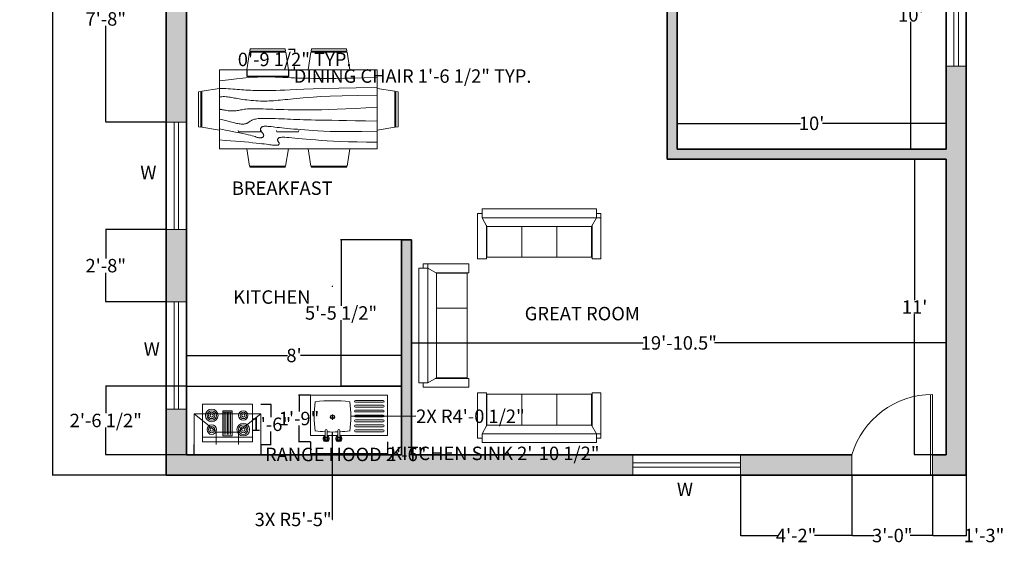
# Model space of a CAD drawing. Units: inches. Extents: x 302 to 1258, y 831 to 1373.
# Tile 1 of 13: x 302 to 742, y 836 to 1070. Entities that reach past the tile are written whole.
import ezdxf

# ---------------------------------------------------------------- set-up
doc = ezdxf.new("R2010")
doc.units = ezdxf.units.IN
doc.header["$MEASUREMENT"] = 0
for name, color, linetype, lineweight in [('A-ANNO-DIMS', 2, 'Continuous', 18), ('A-ANNO-TEXT', 7, 'Continuous', 18), ('A-AREA-IDEN', 7, 'Continuous', 18), ('A-DOOR', 3, 'Continuous', 18), ('A-EQPM', 8, 'Continuous', 18), ('A-FLOR-CASE', 8, 'Continuous', 25), ('A-FLOR-FIXT', 8, 'Continuous', 18), ('A-FURN', 8, 'Continuous', 18), ('A-GLAZ', 4, 'Continuous', 18), ('A-WALL', 7, 'Continuous', 35), ('A-WALL-PATT', 251, 'Continuous', 13)]:
    doc.layers.add(name, color=color, linetype=linetype, lineweight=lineweight)
doc.styles.get("Standard").update_dxf_attribs({"font": 'arial.ttf'})
doc.dimstyles.get("Standard").update_dxf_attribs({"dimtxt": 6, "dimasz": 0.18, "dimexe": 0.18, "dimexo": 0.0625, "dimgap": 0.09, "dimtad": 0, "dimtih": 1, "dimtoh": 1, "dimdec": 1, "dimzin": 0, "dimdsep": 46, "dimlunit": 3, "dimtxsty": 'Standard', "dimcen": 0.09, "dimadec": 0, "dimazin": 0, "dimtfac": 1, "dimtdec": 1, "dimtofl": 0, "dimtmove": 0, "dimatfit": 3, "dimfxl": 1, "dimtolj": 1, "dimtzin": 0, "dimarcsym": 0})

# ---------------------------------------------------------------- blocks, each defined once
blk = doc.blocks.new('chimmne')
for p, q in [((17.89, 6.07), (-18.11, 6.07)), ((-18.11, 6.07), (-18.11, -10.43)), ((-6.16, -3.43), (-18.11, 6.07)), ((5.94, -3.43), (17.89, 6.07)), ((17.89, 6.07), (17.89, -10.43)), ((-6.16, -3.43), (-6.16, -10.43)), ((5.94, -3.82), (-6.16, -3.82)), ((5.94, -3.43), (5.94, -10.43))]:
    blk.add_line(p, q)
for points in [[(-13.61, -9.12), (-13.61, 11.28), (13.39, 11.28), (13.39, -9.12)], [(-2.66, -5.87), (-2.66, 7.73), (2.44, 7.73), (2.44, -5.87)]]:
    blk.add_lwpolyline(points, close=True)
for points in [[(-2.66, 6.88), (2.44, 6.88)], [(-1.81, 6.88), (-1.81, -5.02)], [(-0.96, -5.02), (-0.96, 6.88)], [(-0.11, 6.88), (-0.11, -5.02)], [(0.74, -5.02), (0.74, 6.88)], [(1.59, 6.88), (1.59, -5.02)], [(13.39, -6.57), (-13.61, -6.57)]]:
    blk.add_lwpolyline(points)
for centre, radius in [((-8.55, 5.18), 3.4), ((-8.55, 5.18), 2.55), ((-8.55, 5.18), 1.7), ((-8.55, 5.18), 0.85), ((8.44, 5.18), 2.55), ((8.44, 5.18), 1.7), ((8.44, 5.18), 0.85), ((-8.55, -2.47), 2.55), ((8.44, -2.47), 3.4), ((8.44, -2.47), 2.55), ((-8.55, -2.47), 1.7), ((-8.55, -2.47), 0.85), ((8.44, -2.47), 1.7), ((8.44, -2.47), 0.85)]:
    blk.add_circle(centre, radius)
blk = doc.blocks.new('A$C799204C7')
for p, q in [((0, 34.2), (17.99, 34.2)), ((0, 0), (0, 34.2)), ((2.32, 20.01), (2.32, 32.27)), ((3.13, 20.01), (3.13, 32.27)), ((4.48, 20.01), (4.48, 32.27)), ((5.29, 20.01), (5.29, 32.27)), ((6.64, 20.01), (6.64, 32.27)), ((7.45, 20.01), (7.45, 32.27)), ((8.85, 20.01), (8.85, 32.27)), ((9.66, 20.01), (9.66, 32.27)), ((11.01, 20.01), (11.01, 32.27)), ((11.82, 20.01), (11.82, 32.27)), ((13.22, 20.01), (13.22, 32.27)), ((14.03, 20.01), (14.03, 32.27)), ((15.42, 20.01), (15.42, 32.27)), ((16.24, 20.01), (16.24, 32.27)), ((17.99, 13.08), (17.99, 34.2)), ((8.52, 9.77), (10.9, 9.77)), ((9.73, 11), (9.73, 8.54)), ((18.59, 13.08), (15.71, 13.08)), ((15.71, 12.17), (18.59, 12.17)), ((17.99, 7.36), (17.99, 12.17)), ((18.59, 7.36), (15.71, 7.36)), ((15.71, 6.45), (18.59, 6.45)), ((17.99, 0), (17.99, 6.45)), ((0, 0), (17.99, 0))]:
    blk.add_line(p, q)
for centre, radius in [((19.38, 12.62), 0.684), ((9.7, 9.77), 0.916), ((19.38, 12.62), 0.456), ((19.38, 6.91), 0.684), ((19.38, 6.91), 0.456)]:
    blk.add_circle(centre, radius)
for centre, radius, start, end in [((2.72, 32.27), 0.407, 0, 180), ((4.88, 32.27), 0.407, 0, 180), ((7.05, 32.27), 0.407, 0, 180), ((9.25, 32.27), 0.407, 0, 180), ((11.42, 32.27), 0.407, 0, 180), ((13.62, 32.27), 0.407, 0, 180), ((15.83, 32.27), 0.407, 0, 180), ((2.72, 20.01), 0.407, 180, 0), ((9.53, -30.19), 48.1, 82.3437, 97.8966), ((4.88, 20.01), 0.407, 180, 0), ((7.05, 20.01), 0.407, 180, 0), ((9.25, 20.01), 0.407, 180, 0), ((11.42, 20.01), 0.407, 180, 0), ((13.62, 20.01), 0.407, 180, 0), ((15.83, 20.01), 0.407, 180, 0), ((67.33, 9.77), 64.88, 173.1952, 186.8048), ((-48.51, 9.77), 64.88, 2.9208, 6.8048), ((19.38, 12.62), 1.37, 199.6514, 160.3603), ((19.38, 12.62), 0.911, 210.3431, 149.7554), ((15.71, 12.62), 0.456, 90, 270), ((-48.51, 9.77), 64.88, 357.8723, 2.115), ((15.71, 6.91), 0.456, 90, 270), ((-48.51, 9.77), 64.88, 353.1952, 357.0665), ((19.38, 6.91), 1.37, 199.6514, 160.3603), ((19.38, 6.91), 0.911, 210.3431, 149.7554), ((9.53, 49.73), 48.1, 262.1034, 277.6563)]:
    blk.add_arc(centre, radius, start, end)
blk = doc.blocks.new('*D11')
at = {"layer": 'A-ANNO-DIMS', "color": 0, "lineweight": -2, "transparency": 16777216}
for p, q in [((595.67, 1012.38), (595.67, 1024.04)), ((595.85, 1023.86), (650.77, 1023.86)), ((715.49, 1023.86), (660.57, 1023.86)), ((715.67, 1012.38), (715.67, 1024.04))]:
    blk.add_line(p, q, dxfattribs=at)
at = {"layer": 'A-ANNO-DIMS', "color": 0, "transparency": 16777216}
for points in [[(595.85, 1023.89), (595.85, 1023.83), (595.67, 1023.86)], [(715.49, 1023.89), (715.49, 1023.83), (715.67, 1023.86)]]:
    blk.add_solid(points, dxfattribs=at)
at = {"layer": 'Defpoints', "color": 0, "transparency": 16777216}
for p in [(715.67, 1023.86), (595.67, 1012.32), (715.67, 1012.32)]:
    blk.add_point(p, dxfattribs=at)
at = {"layer": 'A-ANNO-DIMS', "color": 0, "transparency": 16777216, "insert": (655.67, 1023.86), "char_height": 6, "attachment_point": 5}
blk.add_mtext("\\A1;10'", dxfattribs=at)
blk = doc.blocks.new('*D12')
at = {"layer": 'A-ANNO-DIMS', "color": 0, "lineweight": -2, "transparency": 16777216}
for p, q in [((715.61, 1132.32), (699.81, 1132.32)), ((699.99, 1132.14), (699.99, 1075.47)), ((699.99, 1012.5), (699.99, 1069.17)), ((715.61, 1012.32), (699.81, 1012.32))]:
    blk.add_line(p, q, dxfattribs=at)
at = {"layer": 'A-ANNO-DIMS', "color": 0, "transparency": 16777216}
for points in [[(699.96, 1132.14), (700.02, 1132.14), (699.99, 1132.32)], [(699.96, 1012.5), (700.02, 1012.5), (699.99, 1012.32)]]:
    blk.add_solid(points, dxfattribs=at)
at = {"layer": 'Defpoints', "color": 0, "transparency": 16777216}
for p in [(715.67, 1132.32), (699.99, 1012.32), (715.67, 1012.32)]:
    blk.add_point(p, dxfattribs=at)
at = {"layer": 'A-ANNO-DIMS', "color": 0, "transparency": 16777216, "insert": (699.99, 1072.32), "char_height": 6, "attachment_point": 5}
blk.add_mtext("\\A1;10'", dxfattribs=at)
blk = doc.blocks.new('*D13')
at = {"layer": 'A-ANNO-DIMS', "color": 0, "lineweight": -2, "transparency": 16777216}
for p, q in [((376.67, 906.61), (376.67, 920.41)), ((376.85, 920.23), (421.82, 920.23)), ((472.49, 920.23), (427.52, 920.23)), ((472.67, 906.61), (472.67, 920.41))]:
    blk.add_line(p, q, dxfattribs=at)
at = {"layer": 'A-ANNO-DIMS', "color": 0, "transparency": 16777216}
for points in [[(376.85, 920.26), (376.85, 920.2), (376.67, 920.23)], [(472.49, 920.26), (472.49, 920.2), (472.67, 920.23)]]:
    blk.add_solid(points, dxfattribs=at)
at = {"layer": 'Defpoints', "color": 0, "transparency": 16777216}
for p in [(472.67, 920.23), (376.67, 906.55), (472.67, 906.55)]:
    blk.add_point(p, dxfattribs=at)
at = {"layer": 'A-ANNO-DIMS', "color": 0, "transparency": 16777216, "insert": (424.67, 920.23), "char_height": 6, "attachment_point": 5}
blk.add_mtext("\\A1;8'", dxfattribs=at)
blk = doc.blocks.new('*D14')
at = {"layer": 'A-ANNO-DIMS', "color": 0, "lineweight": -2, "transparency": 16777216}
for p, q in [((477.17, 875.88), (477.17, 926)), ((477.35, 925.82), (580.48, 925.82)), ((715.49, 925.82), (612.36, 925.82)), ((715.67, 875.88), (715.67, 926))]:
    blk.add_line(p, q, dxfattribs=at)
at = {"layer": 'A-ANNO-DIMS', "color": 0, "transparency": 16777216}
for points in [[(477.35, 925.85), (477.35, 925.79), (477.17, 925.82)], [(715.49, 925.85), (715.49, 925.79), (715.67, 925.82)]]:
    blk.add_solid(points, dxfattribs=at)
at = {"layer": 'Defpoints', "color": 0, "transparency": 16777216}
for p in [(715.67, 925.82), (477.17, 875.82), (715.67, 875.82)]:
    blk.add_point(p, dxfattribs=at)
at = {"layer": 'A-ANNO-DIMS', "color": 0, "transparency": 16777216, "insert": (596.42, 925.82), "char_height": 6, "attachment_point": 5}
blk.add_mtext('\\A1;19\'-10.5"', dxfattribs=at)
blk = doc.blocks.new('*D15')
at = {"layer": 'A-ANNO-DIMS', "color": 0, "lineweight": -2, "transparency": 16777216}
for p, q in [((715.61, 1007.82), (701.46, 1007.82)), ((701.64, 1007.64), (701.64, 944.92)), ((701.64, 876), (701.64, 938.72)), ((715.61, 875.82), (701.46, 875.82))]:
    blk.add_line(p, q, dxfattribs=at)
at = {"layer": 'A-ANNO-DIMS', "color": 0, "transparency": 16777216}
for points in [[(701.61, 1007.64), (701.67, 1007.64), (701.64, 1007.82)], [(701.61, 876), (701.67, 876), (701.64, 875.82)]]:
    blk.add_solid(points, dxfattribs=at)
at = {"layer": 'Defpoints', "color": 0, "transparency": 16777216}
for p in [(715.67, 1007.82), (701.64, 875.82), (715.67, 875.82)]:
    blk.add_point(p, dxfattribs=at)
at = {"layer": 'A-ANNO-DIMS', "color": 0, "transparency": 16777216, "insert": (701.64, 941.82), "char_height": 6, "attachment_point": 5}
blk.add_mtext("\\A1;11'", dxfattribs=at)
blk = doc.blocks.new('*D32')
at = {"layer": 'A-ANNO-DIMS', "color": 0, "lineweight": -2, "transparency": 16777216}
for p, q in [((367.61, 1342.32), (316.79, 1342.32)), ((316.97, 1342.14), (316.97, 1107.72)), ((316.97, 867), (316.97, 1101.41)), ((367.61, 866.82), (316.79, 866.82))]:
    blk.add_line(p, q, dxfattribs=at)
at = {"layer": 'A-ANNO-DIMS', "color": 0, "transparency": 16777216}
for points in [[(316.94, 1342.14), (317, 1342.14), (316.97, 1342.32)], [(316.94, 867), (317, 867), (316.97, 866.82)]]:
    blk.add_solid(points, dxfattribs=at)
at = {"layer": 'Defpoints', "color": 0, "transparency": 16777216}
for p in [(367.67, 1342.32), (316.97, 866.82), (367.67, 866.82)]:
    blk.add_point(p, dxfattribs=at)
at = {"layer": 'A-ANNO-DIMS', "color": 0, "transparency": 16777216, "insert": (316.97, 1104.57), "char_height": 6, "attachment_point": 5}
blk.add_mtext('\\A1;39\'-7.5"', dxfattribs=at)
blk = doc.blocks.new('SOFA-3-SEAT')
for p, q in [((0, 53.08), (0, 1.96)), ((3.92, 53.08), (0, 53.08)), ((1.96, 55.04), (22.23, 55.04)), ((1.96, 55.04), (1.96, 53.08)), ((3.92, 55.04), (3.92, 1.96)), ((3.92, 53.08), (7.85, 50.88)), ((22.23, 51.12), (22.23, 55.04)), ((7.54, 51.12), (22.23, 51.12)), ((21.57, 50.87), (7.85, 50.87)), ((21.57, 35.3), (7.85, 35.3)), ((21.57, 19.74), (7.85, 19.74)), ((3.92, 1.96), (0, 1.96)), ((1.96, 1.96), (1.96, 0)), ((1.96, 0), (22.23, 0)), ((7.85, 4.17), (3.92, 1.96)), ((7.28, 3.92), (22.23, 3.92)), ((22.23, 3.92), (22.23, 0))]:
    blk.add_line(p, q)
blk.add_lwpolyline([(7.85, 50.88), (7.85, 4.17), (21.57, 4.17), (21.57, 50.87)])
blk = doc.blocks.new('CHAIR-DINING')
for p, q in [((1.3, 8.32), (1.45, 9.3)), ((17.11, 9.3), (1.45, 9.3)), ((17.11, 9.3), (17.26, 8.32)), ((0, 0), (1.22, 7.83)), ((17.33, 7.83), (1.22, 7.83)), ((1.3, 8.32), (17.26, 8.32)), ((17.34, 7.83), (18.56, 0))]:
    blk.add_line(p, q)
blk = doc.blocks.new('WINDOW-48IN')
for p, q in [((0, 0), (0, 9)), ((0, 9), (48, 9)), ((48, 9), (48, 0)), ((0, 5.5), (48, 5.5)), ((48, 3.5), (0, 3.5)), ((48, 0), (0, 0))]:
    blk.add_line(p, q)
blk = doc.blocks.new('*D59')
at = {"layer": 'A-ANNO-DIMS', "color": 0, "lineweight": -2, "transparency": 16777216}
for p, q in [((403.62, 1047.7), (403.62, 1044.8)), ((422.18, 1047.7), (422.18, 1044.8)), ((403.8, 1044.98), (422, 1044.98)), ((422.18, 1044.98), (422.36, 1044.98))]:
    blk.add_line(p, q, dxfattribs=at)
at = {"layer": 'A-ANNO-DIMS', "color": 0, "transparency": 16777216}
for points in [[(403.8, 1045.01), (403.8, 1044.95), (403.62, 1044.98)], [(422, 1045.01), (422, 1044.95), (422.18, 1044.98)]]:
    blk.add_solid(points, dxfattribs=at)
at = {"layer": 'Defpoints', "color": 0, "transparency": 16777216}
for p in [(403.62, 1047.77), (422.18, 1047.77), (422.18, 1044.98)]:
    blk.add_point(p, dxfattribs=at)
at = {"layer": 'A-ANNO-DIMS', "color": 0, "transparency": 16777216, "insert": (477.61, 1044.98), "char_height": 6, "attachment_point": 5}
blk.add_mtext('\\A1;DINING CHAIR 1\'-6 1/2" TYP.', dxfattribs=at)
blk = doc.blocks.new('*D60')
at = {"layer": 'A-ANNO-DIMS', "color": 0, "lineweight": -2, "transparency": 16777216}
for p, q in [((422.24, 1057.06), (425.14, 1057.06)), ((424.96, 1056.88), (424.96, 1055.61)), ((422.24, 1047.77), (425.14, 1047.77)), ((424.96, 1047.95), (424.96, 1049.22))]:
    blk.add_line(p, q, dxfattribs=at)
at = {"layer": 'A-ANNO-DIMS', "color": 0, "transparency": 16777216}
for points in [[(424.93, 1056.88), (424.99, 1056.88), (424.96, 1057.06)], [(424.93, 1047.95), (424.99, 1047.95), (424.96, 1047.77)]]:
    blk.add_solid(points, dxfattribs=at)
at = {"layer": 'Defpoints', "color": 0, "transparency": 16777216}
for p in [(422.18, 1057.06), (424.96, 1057.06), (422.18, 1047.77)]:
    blk.add_point(p, dxfattribs=at)
at = {"layer": 'A-ANNO-DIMS', "color": 0, "transparency": 16777216, "insert": (424.96, 1052.41), "char_height": 6, "attachment_point": 5}
blk.add_mtext('\\A1;0\'-9 1/2" TYP.', dxfattribs=at)
blk = doc.blocks.new('*D65')
at = {"layer": 'A-ANNO-DIMS', "color": 0, "lineweight": -2, "transparency": 16777216}
for p, q in [((380.04, 880.43), (380.04, 875.84)), ((409.85, 880.43), (409.85, 875.84)), ((380.22, 876.02), (409.67, 876.02)), ((409.85, 876.02), (410.03, 876.02))]:
    blk.add_line(p, q, dxfattribs=at)
at = {"layer": 'A-ANNO-DIMS', "color": 0, "transparency": 16777216}
for points in [[(380.22, 876.05), (380.22, 875.99), (380.04, 876.02)], [(409.67, 876.05), (409.67, 875.99), (409.85, 876.02)]]:
    blk.add_solid(points, dxfattribs=at)
at = {"layer": 'Defpoints', "color": 0, "transparency": 16777216}
for p in [(380.04, 880.49), (409.85, 880.49), (409.85, 876.02)]:
    blk.add_point(p, dxfattribs=at)
at = {"layer": 'A-ANNO-DIMS', "color": 0, "transparency": 16777216, "insert": (447.75, 876.02), "char_height": 6, "attachment_point": 5}
blk.add_mtext('\\A1;RANGE HOOD 2\'-6"', dxfattribs=at)
blk = doc.blocks.new('*D66')
at = {"layer": 'A-ANNO-DIMS', "color": 0, "lineweight": -2, "transparency": 16777216}
for p, q in [((409.92, 898.47), (414.51, 898.47)), ((414.33, 898.29), (414.33, 892.63)), ((414.33, 880.67), (414.33, 886.33)), ((409.92, 880.49), (414.51, 880.49))]:
    blk.add_line(p, q, dxfattribs=at)
at = {"layer": 'A-ANNO-DIMS', "color": 0, "transparency": 16777216}
for points in [[(414.3, 898.29), (414.36, 898.29), (414.33, 898.47)], [(414.3, 880.67), (414.36, 880.67), (414.33, 880.49)]]:
    blk.add_solid(points, dxfattribs=at)
at = {"layer": 'Defpoints', "color": 0, "transparency": 16777216}
for p in [(409.85, 898.47), (414.33, 898.47), (409.85, 880.49)]:
    blk.add_point(p, dxfattribs=at)
at = {"layer": 'A-ANNO-DIMS', "color": 0, "transparency": 16777216, "insert": (414.33, 889.48), "char_height": 6, "attachment_point": 5}
blk.add_mtext('\\A1;1\'-6"', dxfattribs=at)
blk = doc.blocks.new('*D67')
at = {"layer": 'A-ANNO-DIMS', "color": 0, "lineweight": -2, "transparency": 16777216}
for p, q in [((432.06, 881.58), (432.06, 876.32)), ((466.37, 881.58), (466.37, 876.32)), ((432.24, 876.5), (466.19, 876.5)), ((466.37, 876.5), (466.55, 876.5))]:
    blk.add_line(p, q, dxfattribs=at)
at = {"layer": 'A-ANNO-DIMS', "color": 0, "transparency": 16777216}
for points in [[(432.24, 876.53), (432.24, 876.47), (432.06, 876.5)], [(466.19, 876.53), (466.19, 876.47), (466.37, 876.5)]]:
    blk.add_solid(points, dxfattribs=at)
at = {"layer": 'Defpoints', "color": 0, "transparency": 16777216}
for p in [(432.06, 881.65), (466.37, 881.65), (466.37, 876.5)]:
    blk.add_point(p, dxfattribs=at)
at = {"layer": 'A-ANNO-DIMS', "color": 0, "transparency": 16777216, "insert": (514.31, 876.5), "char_height": 6, "attachment_point": 5}
blk.add_mtext('\\A1;KITCHEN SINK 2\'-10 1/2"', dxfattribs=at)
blk = doc.blocks.new('*D68')
at = {"layer": 'A-ANNO-DIMS', "color": 0, "lineweight": -2, "transparency": 16777216}
for p, q in [((431.99, 902.46), (426.73, 902.46)), ((426.91, 902.28), (426.91, 895.21)), ((426.91, 881.83), (426.91, 888.9)), ((431.99, 881.65), (426.73, 881.65))]:
    blk.add_line(p, q, dxfattribs=at)
at = {"layer": 'A-ANNO-DIMS', "color": 0, "transparency": 16777216}
for points in [[(426.88, 902.28), (426.94, 902.28), (426.91, 902.46)], [(426.88, 881.83), (426.94, 881.83), (426.91, 881.65)]]:
    blk.add_solid(points, dxfattribs=at)
at = {"layer": 'Defpoints', "color": 0, "transparency": 16777216}
for p in [(432.06, 902.46), (426.91, 881.65), (432.06, 881.65)]:
    blk.add_point(p, dxfattribs=at)
at = {"layer": 'A-ANNO-DIMS', "color": 0, "transparency": 16777216, "insert": (426.91, 892.05), "char_height": 6, "attachment_point": 5}
blk.add_mtext('\\A1;1\'-9"', dxfattribs=at)
blk = doc.blocks.new('*D73')
at = {"layer": 'A-ANNO-DIMS', "color": 0, "lineweight": -2, "transparency": 16777216}
for p, q in [((367.61, 1116.55), (340.49, 1116.55)), ((340.67, 1116.37), (340.67, 1073.65)), ((340.67, 1024.62), (340.67, 1067.34)), ((367.61, 1024.44), (340.49, 1024.44))]:
    blk.add_line(p, q, dxfattribs=at)
at = {"layer": 'A-ANNO-DIMS', "color": 0, "transparency": 16777216}
for points in [[(340.64, 1116.37), (340.7, 1116.37), (340.67, 1116.55)], [(340.64, 1024.62), (340.7, 1024.62), (340.67, 1024.44)]]:
    blk.add_solid(points, dxfattribs=at)
at = {"layer": 'Defpoints', "color": 0, "transparency": 16777216}
for p in [(367.67, 1116.55), (340.67, 1024.44), (367.67, 1024.44)]:
    blk.add_point(p, dxfattribs=at)
at = {"layer": 'A-ANNO-DIMS', "color": 0, "transparency": 16777216, "insert": (340.67, 1070.49), "char_height": 6, "attachment_point": 5}
blk.add_mtext('\\A1;7\'-8"', dxfattribs=at)
blk = doc.blocks.new('*D74')
at = {"layer": 'A-ANNO-DIMS', "color": 0, "lineweight": -2, "transparency": 16777216}
for p, q in [((367.61, 976.44), (340.49, 976.44)), ((340.67, 976.26), (340.67, 963.47)), ((340.67, 944.38), (340.67, 957.17)), ((367.61, 944.2), (340.49, 944.2))]:
    blk.add_line(p, q, dxfattribs=at)
at = {"layer": 'A-ANNO-DIMS', "color": 0, "transparency": 16777216}
for points in [[(340.64, 976.26), (340.7, 976.26), (340.67, 976.44)], [(340.64, 944.38), (340.7, 944.38), (340.67, 944.2)]]:
    blk.add_solid(points, dxfattribs=at)
at = {"layer": 'Defpoints', "color": 0, "transparency": 16777216}
for p in [(367.67, 976.44), (340.67, 944.2), (367.67, 944.2)]:
    blk.add_point(p, dxfattribs=at)
at = {"layer": 'A-ANNO-DIMS', "color": 0, "transparency": 16777216, "insert": (340.67, 960.32), "char_height": 6, "attachment_point": 5}
blk.add_mtext('\\A1;2\'-8"', dxfattribs=at)
blk = doc.blocks.new('*D78')
at = {"layer": 'A-ANNO-DIMS', "color": 0, "lineweight": -2, "transparency": 16777216}
for p, q in [((623.88, 866.76), (623.88, 839.64)), ((673.67, 866.76), (673.67, 839.64)), ((624.06, 839.82), (640.59, 839.82)), ((673.49, 839.82), (656.96, 839.82))]:
    blk.add_line(p, q, dxfattribs=at)
at = {"layer": 'A-ANNO-DIMS', "color": 0, "transparency": 16777216}
for points in [[(624.06, 839.85), (624.06, 839.79), (623.88, 839.82)], [(673.49, 839.85), (673.49, 839.79), (673.67, 839.82)]]:
    blk.add_solid(points, dxfattribs=at)
at = {"layer": 'Defpoints', "color": 0, "transparency": 16777216}
for p in [(623.88, 866.82), (673.67, 866.82), (673.67, 839.82)]:
    blk.add_point(p, dxfattribs=at)
at = {"layer": 'A-ANNO-DIMS', "color": 0, "transparency": 16777216, "insert": (648.77, 839.82), "char_height": 6, "attachment_point": 5}
blk.add_mtext('\\A1;4\'-2"', dxfattribs=at)
blk = doc.blocks.new('*D79')
at = {"layer": 'A-ANNO-DIMS', "color": 0, "lineweight": -2, "transparency": 16777216}
for p, q in [((673.67, 866.76), (673.67, 839.64)), ((709.67, 866.76), (709.67, 839.64)), ((673.85, 839.82), (683.61, 839.82)), ((709.49, 839.82), (699.73, 839.82))]:
    blk.add_line(p, q, dxfattribs=at)
at = {"layer": 'A-ANNO-DIMS', "color": 0, "transparency": 16777216}
for points in [[(673.85, 839.85), (673.85, 839.79), (673.67, 839.82)], [(709.49, 839.85), (709.49, 839.79), (709.67, 839.82)]]:
    blk.add_solid(points, dxfattribs=at)
at = {"layer": 'Defpoints', "color": 0, "transparency": 16777216}
for p in [(673.67, 866.82), (709.67, 866.82), (709.67, 839.82)]:
    blk.add_point(p, dxfattribs=at)
at = {"layer": 'A-ANNO-DIMS', "color": 0, "transparency": 16777216, "insert": (691.67, 839.82), "char_height": 6, "attachment_point": 5}
blk.add_mtext('\\A1;3\'-0"', dxfattribs=at)
blk = doc.blocks.new('*D80')
at = {"layer": 'A-ANNO-DIMS', "color": 0, "lineweight": -2, "transparency": 16777216}
for p, q in [((709.67, 866.76), (709.67, 839.64)), ((724.67, 866.76), (724.67, 839.64)), ((709.85, 839.82), (724.49, 839.82)), ((724.67, 839.82), (724.85, 839.82))]:
    blk.add_line(p, q, dxfattribs=at)
at = {"layer": 'A-ANNO-DIMS', "color": 0, "transparency": 16777216}
for points in [[(709.85, 839.85), (709.85, 839.79), (709.67, 839.82)], [(724.49, 839.85), (724.49, 839.79), (724.67, 839.82)]]:
    blk.add_solid(points, dxfattribs=at)
at = {"layer": 'Defpoints', "color": 0, "transparency": 16777216}
for p in [(709.67, 866.82), (724.67, 866.82), (724.67, 839.82)]:
    blk.add_point(p, dxfattribs=at)
at = {"layer": 'A-ANNO-DIMS', "color": 0, "transparency": 16777216, "insert": (732.63, 839.82), "char_height": 6, "attachment_point": 5}
blk.add_mtext('\\A1;1\'-3"', dxfattribs=at)
blk = doc.blocks.new('*D81')
at = {"layer": 'A-ANNO-DIMS', "color": 0, "lineweight": -2, "transparency": 16777216}
for p, q in [((472.61, 971.82), (445.49, 971.82)), ((445.67, 971.64), (445.67, 942.38)), ((445.67, 906.73), (445.67, 935.99)), ((472.61, 906.55), (445.49, 906.55))]:
    blk.add_line(p, q, dxfattribs=at)
at = {"layer": 'A-ANNO-DIMS', "color": 0, "transparency": 16777216}
for points in [[(445.64, 971.64), (445.7, 971.64), (445.67, 971.82)], [(445.64, 906.73), (445.7, 906.73), (445.67, 906.55)]]:
    blk.add_solid(points, dxfattribs=at)
at = {"layer": 'Defpoints', "color": 0, "transparency": 16777216}
for p in [(445.67, 971.82), (472.67, 971.82), (472.67, 906.55)]:
    blk.add_point(p, dxfattribs=at)
at = {"layer": 'A-ANNO-DIMS', "color": 0, "transparency": 16777216, "insert": (445.67, 939.19), "char_height": 6, "attachment_point": 5}
blk.add_mtext('\\A1;5\'-5 1/2"', dxfattribs=at)
blk = doc.blocks.new('*D82')
at = {"layer": 'A-ANNO-DIMS', "color": 0, "lineweight": -2, "transparency": 16777216}
for p, q in [((376.61, 906.55), (340.49, 906.55)), ((340.67, 906.37), (340.67, 894.38)), ((340.67, 876), (340.67, 887.99)), ((376.61, 875.82), (340.49, 875.82))]:
    blk.add_line(p, q, dxfattribs=at)
at = {"layer": 'A-ANNO-DIMS', "color": 0, "transparency": 16777216}
for points in [[(340.64, 906.37), (340.7, 906.37), (340.67, 906.55)], [(340.64, 876), (340.7, 876), (340.67, 875.82)]]:
    blk.add_solid(points, dxfattribs=at)
at = {"layer": 'Defpoints', "color": 0, "transparency": 16777216}
for p in [(340.67, 906.55), (376.67, 906.55), (376.67, 875.82)]:
    blk.add_point(p, dxfattribs=at)
at = {"layer": 'A-ANNO-DIMS', "color": 0, "transparency": 16777216, "insert": (340.67, 891.19), "char_height": 6, "attachment_point": 5}
blk.add_mtext('\\A1;2\'-6 1/2"', dxfattribs=at)
blk = doc.blocks.new('*D98')
at = {"layer": 'A-ANNO-DIMS', "color": 0, "lineweight": -2, "transparency": 16777216}
for p, q in [((441.77, 951.13), (441.95, 951.13)), ((441.86, 951.04), (441.86, 951.22)), ((441.85, 846.99), (441.85, 885.86)), ((441.67, 846.99), (441.85, 846.99))]:
    blk.add_line(p, q, dxfattribs=at)
at = {"layer": 'A-ANNO-DIMS', "color": 0, "transparency": 16777216}
blk.add_solid([(441.82, 885.86), (441.88, 885.86), (441.85, 886.04)], dxfattribs=at)
at = {"layer": 'Defpoints', "color": 0, "transparency": 16777216}
for p in [(441.86, 951.13), (441.85, 886.04)]:
    blk.add_point(p, dxfattribs=at)
at = {"layer": 'A-ANNO-DIMS', "color": 0, "transparency": 16777216, "insert": (424.29, 846.99), "char_height": 6, "attachment_point": 5}
blk.add_mtext('\\A1;3X R5\'-5"', dxfattribs=at)
blk = doc.blocks.new('*D99')
at = {"layer": 'A-ANNO-DIMS', "color": 0, "lineweight": -2, "transparency": 16777216}
for p, q in [((401.68, 892.9), (401.86, 892.9)), ((401.77, 892.81), (401.77, 892.99)), ((478.98, 893.07), (450.21, 893.01))]:
    blk.add_line(p, q, dxfattribs=at)
at = {"layer": 'A-ANNO-DIMS', "color": 0, "transparency": 16777216}
blk.add_solid([(450.21, 893.04), (450.21, 892.98), (450.03, 893.01)], dxfattribs=at)
at = {"layer": 'Defpoints', "color": 0, "transparency": 16777216}
for p in [(401.77, 892.9), (450.03, 893.01)]:
    blk.add_point(p, dxfattribs=at)
at = {"layer": 'A-ANNO-DIMS', "color": 0, "transparency": 16777216, "insert": (503.41, 893.07), "char_height": 6, "attachment_point": 5}
blk.add_mtext('\\A1;2X R4\'-0 1/2"', dxfattribs=at)

msp = doc.modelspace()

# ---------------------------------------------------------------- hatches: boundary and pattern name
at = {"layer": 'A-WALL-PATT'}
h = msp.add_hatch(color=256, dxfattribs=at)
h.dxf.hatch_style = 1
h.paths.add_polyline_path([(524.78, 1342.32), (455.57, 1342.32), (455.57, 1333.32), (496.67, 1333.32), (496.67, 1330.32), (501.17, 1330.32), (501.17, 1333.32), (524.78, 1333.32)])
h.paths.add_polyline_path([(724.67, 1342.32), (548.78, 1342.32), (548.78, 1333.32), (567.17, 1333.32), (567.17, 1213.32), (501.17, 1213.32), (501.17, 1306.32), (496.67, 1306.32), (496.67, 1213.32), (495.67, 1213.32), (495.67, 1208.82), (496.67, 1208.82), (572.67, 1208.82), (572.67, 1213.32), (571.67, 1213.32), (571.67, 1333.32), (715.67, 1333.32), (715.67, 1302.71), (724.67, 1302.71)])
h.paths.add_polyline_path([(376.67, 1333.32), (407.57, 1333.32), (407.57, 1342.32), (367.67, 1342.32), (367.67, 1300.76), (376.67, 1300.76)])
h.paths.add_polyline_path([(459.67, 1213.32), (376.67, 1213.32), (376.67, 1252.76), (367.67, 1252.76), (367.67, 1164.55), (376.67, 1164.55), (376.67, 1208.82), (454.67, 1208.82), (454.67, 1082.82), (459.17, 1082.82), (459.17, 1208.82), (459.67, 1208.82)])
h.paths.add_polyline_path([(376.67, 1116.55), (367.67, 1116.55), (367.67, 1024.44), (376.67, 1024.44)])
h.paths.add_polyline_path([(724.67, 1254.71), (715.67, 1254.71), (715.67, 1213.32), (608.67, 1213.32), (608.67, 1208.82), (615.17, 1208.82), (615.17, 1205.82), (619.67, 1205.82), (619.67, 1208.82), (715.67, 1208.82), (715.67, 1191.3), (724.67, 1191.3)])
h.paths.add_polyline_path([(724.67, 1167.3), (715.67, 1167.3), (715.67, 1136.82), (619.67, 1136.82), (619.67, 1181.82), (615.17, 1181.82), (615.17, 1136.82), (591.17, 1136.82), (591.17, 1129.32), (595.67, 1129.32), (595.67, 1132.32), (715.67, 1132.32), (715.67, 1097.42), (724.67, 1097.42)])
h.paths.add_polyline_path([(724.67, 1049.42), (715.67, 1049.42), (715.67, 1012.32), (595.67, 1012.32), (595.67, 1093.32), (591.17, 1093.32), (591.17, 1007.82), (715.67, 1007.82), (715.67, 875.82), (709.67, 875.82), (709.67, 866.82), (715.67, 866.82), (724.67, 866.82)])
h.paths.add_polyline_path([(673.67, 875.82), (623.88, 875.82), (623.88, 866.82), (673.67, 866.82)], flags=17)
h.paths.add_polyline_path([(575.88, 875.82), (477.17, 875.82), (477.17, 971.82), (472.67, 971.82), (472.67, 875.82), (376.67, 875.82), (376.67, 896.2), (367.67, 896.2), (367.67, 866.82), (575.88, 866.82)])
h.paths.add_polyline_path([(376.67, 976.44), (367.67, 976.44), (367.67, 944.2), (376.67, 944.2)])

# ---------------------------------------------------------------- linework, layer by layer
at = {"layer": 'A-DOOR'}
for p, q in [((708.67, 902.82), (708.67, 866.82)), ((709.67, 866.82), (709.67, 902.82)), ((709.67, 902.82), (709.67, 866.82)), ((673.67, 866.82), (673.67, 875.82)), ((709.67, 866.82), (673.67, 866.82)), ((715.67, 866.82), (709.67, 866.82))]:
    msp.add_line(p, q, dxfattribs=at)
msp.add_arc((709.67, 865.32), 37.5, 90, 163.7398, dxfattribs=at)
at = {"layer": 'A-FLOR-CASE'}
msp.add_line((376.67, 906.55), (472.67, 906.55), dxfattribs=at)
at = {"layer": 'A-FURN'}
for p, q in [((461.82, 1047.77), (391.37, 1047.77)), ((391.37, 1047.77), (391.37, 1012.54)), ((461.82, 1012.54), (461.82, 1047.77)), ((383.05, 1038.14), (382.08, 1037.98)), ((382.08, 1022.33), (382.08, 1037.98)), ((383.05, 1038.14), (383.05, 1022.18)), ((391.37, 1039.44), (383.54, 1038.21)), ((383.54, 1022.1), (383.54, 1038.22)), ((461.82, 1039.44), (469.64, 1038.21)), ((469.65, 1022.1), (469.65, 1038.22)), ((470.13, 1038.14), (470.13, 1022.18)), ((470.13, 1038.14), (471.11, 1037.98)), ((471.11, 1022.33), (471.11, 1037.98)), ((382.08, 1022.33), (383.05, 1022.18)), ((383.54, 1022.1), (391.37, 1020.88)), ((399.81, 1020.62), (399.91, 1020.01)), ((409.67, 1020.01), (399.91, 1020.01)), ((409.67, 1020.01), (409.76, 1020.62)), ((416.89, 1020.62), (416.99, 1020.01)), ((426.75, 1020.01), (416.99, 1020.01)), ((426.75, 1020.01), (426.84, 1020.62)), ((469.65, 1022.1), (461.82, 1020.88)), ((471.11, 1022.33), (470.13, 1022.18)), ((391.37, 1012.54), (461.82, 1012.54)), ((403.62, 1012.55), (404.84, 1004.72)), ((420.95, 1004.72), (422.18, 1012.55)), ((431.01, 1012.55), (432.24, 1004.72)), ((448.35, 1004.72), (449.57, 1012.55)), ((420.95, 1004.72), (404.83, 1004.72)), ((404.91, 1004.23), (420.87, 1004.23)), ((448.34, 1004.72), (432.23, 1004.72)), ((432.31, 1004.23), (448.27, 1004.23))]:
    msp.add_line(p, q, dxfattribs=at)
for points in [[(461.82, 1044.34), (456.03, 1044.18), (451.09, 1044.06), (446.88, 1043.98), (443.3, 1043.93), (440.26, 1043.9), (437.65, 1043.9), (435.37, 1043.91), (433.32, 1043.94), (431.41, 1043.97), (429.62, 1044.01), (427.94, 1044.06), (426.35, 1044.11), (424.87, 1044.16), (423.47, 1044.22), (422.14, 1044.28), (420.89, 1044.34), (419.69, 1044.4), (418.54, 1044.46), (417.4, 1044.52), (416.27, 1044.56), (415.13, 1044.6), (413.94, 1044.62), (412.7, 1044.64), (411.39, 1044.63), (409.97, 1044.6), (408.38, 1044.54), (406.56, 1044.44), (404.42, 1044.29), (401.91, 1044.06), (398.94, 1043.76), (395.45, 1043.37), (391.37, 1042.88)], [(461.82, 1039.94), (452.43, 1039.76), (444.66, 1039.58), (438.32, 1039.4), (433.19, 1039.24), (429.06, 1039.08), (425.73, 1038.94), (423, 1038.82), (420.64, 1038.72), (418.5, 1038.64), (416.51, 1038.58), (414.69, 1038.54), (413, 1038.51), (411.44, 1038.51), (410, 1038.51), (408.67, 1038.53), (407.43, 1038.55), (406.28, 1038.59), (405.2, 1038.63), (404.17, 1038.68), (403.18, 1038.73), (402.22, 1038.79), (401.28, 1038.86), (400.33, 1038.93), (399.36, 1039), (398.37, 1039.08), (397.36, 1039.16), (396.33, 1039.23), (395.3, 1039.3), (394.29, 1039.36), (393.28, 1039.41), (392.31, 1039.44), (391.37, 1039.45)], [(461.82, 1036.52), (453.19, 1036.33), (446.24, 1036.15), (440.75, 1035.97), (436.49, 1035.79), (433.22, 1035.62), (430.74, 1035.45), (428.81, 1035.29), (427.21, 1035.13), (425.74, 1034.98), (424.37, 1034.84), (423.08, 1034.71), (421.87, 1034.58), (420.72, 1034.46), (419.62, 1034.35), (418.57, 1034.25), (417.54, 1034.15), (416.54, 1034.06), (415.56, 1033.99), (414.59, 1033.92), (413.63, 1033.87), (412.67, 1033.83), (411.7, 1033.81), (410.71, 1033.81), (409.72, 1033.83), (408.7, 1033.87), (407.67, 1033.93), (406.63, 1034.01), (405.61, 1034.1), (404.6, 1034.21), (403.63, 1034.32), (402.69, 1034.44), (401.81, 1034.56), (400.98, 1034.68), (400.21, 1034.8), (399.48, 1034.92), (398.79, 1035.04), (398.12, 1035.16), (397.48, 1035.28), (396.85, 1035.39), (396.22, 1035.5), (395.59, 1035.6), (394.96, 1035.69), (394.34, 1035.76), (393.72, 1035.81), (393.11, 1035.82), (392.51, 1035.78), (391.93, 1035.69), (391.37, 1035.54)], [(461.82, 1031.13), (456.72, 1030.8), (452.05, 1030.53), (447.78, 1030.32), (443.87, 1030.15), (440.29, 1030.03), (437.02, 1029.95), (434.01, 1029.9), (431.24, 1029.87), (428.68, 1029.86), (426.31, 1029.88), (424.12, 1029.9), (422.08, 1029.94), (420.18, 1029.98), (418.41, 1030.04), (416.75, 1030.1), (415.18, 1030.16), (413.69, 1030.22), (412.28, 1030.27), (410.94, 1030.33), (409.69, 1030.37), (408.51, 1030.4), (407.42, 1030.42), (406.4, 1030.42), (405.48, 1030.4), (404.63, 1030.36), (403.86, 1030.3), (403.16, 1030.22), (402.51, 1030.14), (401.91, 1030.04), (401.36, 1029.94), (400.84, 1029.84), (400.34, 1029.75), (399.86, 1029.66), (399.38, 1029.58), (398.91, 1029.52), (398.44, 1029.46), (397.96, 1029.43), (397.47, 1029.4), (396.96, 1029.4), (396.43, 1029.42), (395.86, 1029.46), (395.28, 1029.52), (394.71, 1029.6), (394.15, 1029.68), (393.62, 1029.76), (393.14, 1029.85), (392.73, 1029.93), (392.39, 1029.99), (392.14, 1030.05), (391.97, 1030.09), (391.86, 1030.12), (391.77, 1030.14), (391.7, 1030.15), (391.63, 1030.15), (391.52, 1030.16), (391.37, 1030.16)], [(461.82, 1024.78), (456.65, 1024.94), (452.1, 1025.06), (448.11, 1025.15), (444.62, 1025.21), (441.56, 1025.26), (438.87, 1025.29), (436.49, 1025.32), (434.34, 1025.35), (432.38, 1025.38), (430.57, 1025.42), (428.89, 1025.47), (427.32, 1025.52), (425.84, 1025.57), (424.42, 1025.63), (423.05, 1025.69), (421.7, 1025.75), (420.36, 1025.81), (419.03, 1025.87), (417.72, 1025.93), (416.44, 1025.98), (415.21, 1026.02), (414.04, 1026.05), (412.94, 1026.07), (411.92, 1026.08), (410.98, 1026.07), (410.14, 1026.05), (409.37, 1026.01), (408.69, 1025.96), (408.07, 1025.89), (407.53, 1025.8), (407.04, 1025.71), (406.62, 1025.59), (406.25, 1025.46), (405.92, 1025.32), (405.63, 1025.17), (405.37, 1025.01), (405.14, 1024.85), (404.92, 1024.68), (404.71, 1024.52), (404.5, 1024.37), (404.28, 1024.22), (404.05, 1024.08), (403.81, 1023.95), (403.55, 1023.84), (403.27, 1023.74), (402.97, 1023.66), (402.65, 1023.59), (402.3, 1023.55), (401.91, 1023.53), (401.51, 1023.54), (401.07, 1023.56), (400.61, 1023.6), (400.14, 1023.67), (399.65, 1023.75), (399.14, 1023.85), (398.63, 1023.96), (398.1, 1024.09), (397.53, 1024.24), (396.88, 1024.41), (396.13, 1024.61), (395.24, 1024.84), (394.17, 1025.11), (392.89, 1025.41), (391.37, 1025.75)], [(461.82, 1020.37), (454.95, 1020.23), (449.27, 1020.17), (444.62, 1020.18), (440.85, 1020.24), (437.79, 1020.34), (435.28, 1020.48), (433.16, 1020.63), (431.28, 1020.78), (429.5, 1020.93), (427.79, 1021.07), (426.16, 1021.21), (424.61, 1021.34), (423.14, 1021.47), (421.76, 1021.59), (420.46, 1021.72), (419.26, 1021.84), (418.14, 1021.96), (417.11, 1022.08), (416.17, 1022.19), (415.31, 1022.3), (414.53, 1022.39), (413.83, 1022.47), (413.21, 1022.53), (412.65, 1022.57), (412.16, 1022.59), (411.74, 1022.59), (411.38, 1022.57), (411.06, 1022.52), (410.79, 1022.46), (410.56, 1022.38), (410.37, 1022.28), (410.21, 1022.17), (410.06, 1022.04), (409.95, 1021.89), (409.85, 1021.74), (409.79, 1021.57), (409.75, 1021.4), (409.74, 1021.23), (409.75, 1021.04), (409.8, 1020.86), (409.87, 1020.68), (409.97, 1020.49), (410.09, 1020.31), (410.23, 1020.13), (410.37, 1019.94), (410.51, 1019.76), (410.65, 1019.58), (410.78, 1019.39), (410.89, 1019.21), (410.99, 1019.03), (411.06, 1018.85), (411.11, 1018.67), (411.14, 1018.5), (411.13, 1018.33), (411.09, 1018.16), (411.02, 1018.01), (410.91, 1017.86), (410.76, 1017.72), (410.59, 1017.6), (410.38, 1017.5), (410.14, 1017.42), (409.89, 1017.37), (409.61, 1017.34), (409.31, 1017.36), (408.99, 1017.4), (408.65, 1017.49), (408.26, 1017.6), (407.82, 1017.75), (407.3, 1017.92), (406.7, 1018.11), (406, 1018.31), (405.19, 1018.54), (404.25, 1018.77), (403.15, 1019.03), (401.86, 1019.31), (400.34, 1019.62), (398.57, 1019.98), (396.51, 1020.38), (394.12, 1020.83), (391.37, 1021.35)], [(461.82, 1015.48), (457.1, 1015.5), (452.82, 1015.56), (448.95, 1015.66), (445.45, 1015.79), (442.28, 1015.93), (439.41, 1016.1), (436.79, 1016.28), (434.38, 1016.46), (432.16, 1016.64), (430.12, 1016.82), (428.25, 1016.99), (426.56, 1017.15), (425.03, 1017.3), (423.68, 1017.42), (422.49, 1017.52), (421.46, 1017.6), (420.59, 1017.65), (419.86, 1017.66), (419.27, 1017.65), (418.79, 1017.62), (418.41, 1017.56), (418.11, 1017.49), (417.88, 1017.39), (417.71, 1017.27), (417.57, 1017.14), (417.47, 1017), (417.41, 1016.85), (417.37, 1016.69), (417.36, 1016.53), (417.37, 1016.37), (417.41, 1016.21), (417.46, 1016.05), (417.53, 1015.9), (417.61, 1015.76), (417.69, 1015.62), (417.78, 1015.49), (417.86, 1015.36), (417.93, 1015.24), (417.99, 1015.11), (418.03, 1014.99), (418.05, 1014.87), (418.05, 1014.75), (418.02, 1014.63), (417.97, 1014.52), (417.9, 1014.42), (417.8, 1014.33), (417.68, 1014.24), (417.54, 1014.18), (417.38, 1014.12), (417.18, 1014.08), (416.96, 1014.06), (416.69, 1014.05), (416.37, 1014.06), (416.01, 1014.08), (415.58, 1014.12), (415.1, 1014.18), (414.54, 1014.24), (413.9, 1014.33), (413.17, 1014.42), (412.34, 1014.53), (411.39, 1014.65), (410.31, 1014.78), (409.09, 1014.92), (407.72, 1015.07), (406.18, 1015.23), (404.49, 1015.39), (402.65, 1015.56), (400.66, 1015.73), (398.53, 1015.91), (396.27, 1016.09), (393.88, 1016.28), (391.37, 1016.46)]]:
    msp.add_lwpolyline(points, dxfattribs=at)
at = {"layer": 'A-WALL'}
for p, q in [((367.67, 1342.32), (367.67, 866.82)), ((724.67, 1342.32), (724.67, 866.82)), ((376.67, 1208.82), (376.67, 875.82)), ((591.17, 1136.82), (591.17, 1007.82)), ((715.67, 1132.32), (715.67, 1012.32)), ((595.67, 1093.32), (595.67, 1012.32)), ((595.67, 1012.32), (715.67, 1012.32)), ((591.17, 1007.82), (715.67, 1007.82)), ((715.67, 1007.82), (715.67, 875.82)), ((472.67, 971.82), (472.67, 875.82)), ((472.67, 971.82), (477.17, 971.82)), ((477.17, 971.82), (477.17, 875.82)), ((376.67, 875.82), (472.67, 875.82)), ((477.17, 875.82), (673.67, 875.82)), ((709.67, 875.82), (715.67, 875.82)), ((367.67, 866.82), (724.67, 866.82))]:
    msp.add_line(p, q, dxfattribs=at)

# ---------------------------------------------------------------- block references
at = {"layer": 'A-EQPM', "xscale": 0.8280321260258986, "yscale": 0.8280321260258986, "zscale": 0.8280321260258986}
msp.add_blockref('chimmne', (395.04, 889.13), dxfattribs=at)
at = {"layer": 'A-FLOR-FIXT', "xscale": 1.0032, "yscale": 1.0032, "zscale": 1.0032, "rotation": 270}
msp.add_blockref('A$C799204C7', (432.06, 902.46), dxfattribs=at)
at = {"layer": 'A-FURN'}
for name, p in [('CHAIR-DINING', (403.62, 1047.77)), ('CHAIR-DINING', (431.01, 1047.77)), ('SOFA-3-SEAT', (480.42, 906.05))]:
    msp.add_blockref(name, p, dxfattribs=at)
at = {"layer": 'A-FURN', "rotation": 269.9999999999989}
msp.add_blockref('SOFA-3-SEAT', (506.63, 985.64), dxfattribs=at)
at = {"layer": 'A-FURN', "extrusion": (0, 0, -1), "zscale": -1, "rotation": 90.00000000000087}
msp.add_blockref('SOFA-3-SEAT', (-506.63, 881.3), dxfattribs=at)
at = {"layer": 'A-GLAZ'}
for p, rotation in [((715.67, 1097.42), 269.9999999999995), ((376.67, 976.44), 89.99999999999935), ((376.67, 896.2), 89.99999999999945), ((623.88, 875.82), 180)]:
    msp.add_blockref('WINDOW-48IN', p, dxfattribs=dict(at, rotation=rotation))

# ---------------------------------------------------------------- texts
at = {"layer": 'A-ANNO-TEXT', "char_height": 6, "attachment_point": 1}
for insert in [(356.08, 1004.91), (357.6, 926.07), (595.56, 863.39)]:
    msp.add_mtext_dynamic_manual_height_columns('W', width=16.4894, gutter_width=30, heights=[0], dxfattribs=dict(at, insert=insert))
at = {"layer": 'A-AREA-IDEN', "char_height": 6, "attachment_point": 1}
for s, width, insert in [('BREAKFAST', 56.2165, (396.96, 997.92)), ('KITCHEN', 54.2367, (397.53, 949.3)), ('GREAT ROOM', 70.159, (527.63, 941.9))]:
    msp.add_mtext_dynamic_manual_height_columns(s, width=width, gutter_width=30, heights=[0], dxfattribs=dict(at, insert=insert))

# ---------------------------------------------------------------- dimensions: what is measured, and where the dimension line sits
at = {"layer": 'A-ANNO-DIMS'}
for base, p1, p2, angle, override, picture, middle in [((316.97, 866.82), (367.67, 1342.32), (367.67, 866.82), 90, {"dimclrd": 0, "dimclre": 0, "dimclrt": 0}, '*D32', (316.97, 1104.57)), ((699.99, 1012.32), (715.67, 1132.32), (715.67, 1012.32), 90, {"dimclrd": 0, "dimclre": 0, "dimclrt": 0}, '*D12', (699.99, 1072.32)), ((340.67, 1024.44), (367.67, 1116.55), (367.67, 1024.44), 90, {"dimdec": 1, "dimlfac": 1, "dimrnd": 0, "dimzin": 1, "dimdsep": 46, "dimlunit": 4, "dimfrac": 2}, '*D73', (340.67, 1070.49)), ((701.64, 875.82), (715.67, 1007.82), (715.67, 875.82), 90, {"dimclrd": 0, "dimclre": 0, "dimclrt": 0}, '*D15', (701.64, 941.82)), ((340.67, 944.2), (367.67, 976.44), (367.67, 944.2), 90, {"dimdec": 1, "dimlfac": 1, "dimrnd": 0, "dimzin": 1, "dimdsep": 46, "dimlunit": 4, "dimfrac": 2}, '*D74', (340.67, 960.32)), ((445.67, 971.82), (472.67, 906.55), (472.67, 971.82), 90, {"dimdec": 1, "dimlfac": 1, "dimrnd": 0, "dimzin": 1, "dimdsep": 46, "dimlunit": 4, "dimfrac": 2}, '*D81', (445.67, 939.19)), ((340.67, 906.55), (376.67, 875.82), (376.67, 906.55), 90, {"dimdec": 1, "dimlfac": 1, "dimrnd": 0, "dimzin": 1, "dimdsep": 46, "dimlunit": 4, "dimfrac": 2}, '*D82', (340.67, 891.19)), ((426.91, 881.65), (432.06, 902.46), (432.06, 881.65), 270, {"dimdec": 1, "dimlfac": 1, "dimrnd": 0, "dimzin": 1, "dimdsep": 46, "dimlunit": 4, "dimfrac": 2}, '*D68', (426.91, 892.05)), ((414.33, 898.47), (409.85, 880.49), (409.85, 898.47), 90, {"dimdec": 1, "dimlfac": 1, "dimrnd": 0, "dimzin": 1, "dimdsep": 46, "dimlunit": 4, "dimfrac": 2}, '*D66', (414.33, 889.48))]:
    dim = msp.add_linear_dim(base=base, p1=p1, p2=p2, angle=angle, dimstyle='Standard', override=override, dxfattribs=at)
    dim.commit()
    dim.dimension.update_dxf_attribs({"geometry": picture, "text_midpoint": middle})
for base, p1, p2, text, picture, middle in [((422.18, 1044.98), (403.62, 1047.77), (422.18, 1047.77), 'DINING CHAIR <> TYP.', '*D59', (477.61, 1044.98)), ((466.37, 876.5), (432.06, 881.65), (466.37, 881.65), 'KITCHEN SINK <>', '*D67', (514.31, 876.5)), ((409.85, 876.02), (380.04, 880.49), (409.85, 880.49), 'RANGE HOOD <>', '*D65', (447.75, 876.02))]:
    dim = msp.add_linear_dim(base=base, p1=p1, p2=p2, text=text, dimstyle='Standard', override={"dimdec": 1, "dimlfac": 1, "dimrnd": 0, "dimzin": 1, "dimdsep": 46, "dimlunit": 4, "dimfrac": 2}, dxfattribs=at)
    dim.commit()
    dim.dimension.update_dxf_attribs({"geometry": picture, "text_midpoint": middle})
dim = msp.add_linear_dim(base=(424.96, 1057.06), p1=(422.18, 1047.77), p2=(422.18, 1057.06), angle=90, text='<> TYP.', dimstyle='Standard', override={"dimdec": 1, "dimlfac": 1, "dimrnd": 0, "dimzin": 1, "dimdsep": 46, "dimlunit": 4, "dimfrac": 2}, dxfattribs=at)
dim.commit()
dim.dimension.update_dxf_attribs({"geometry": '*D60', "text_midpoint": (424.96, 1052.41)})
for base, p1, p2, override, picture, middle in [((715.67, 1023.86), (595.67, 1012.32), (715.67, 1012.32), {"dimclrd": 0, "dimclre": 0, "dimclrt": 0}, '*D11', (655.67, 1023.86)), ((715.67, 925.82), (477.17, 875.82), (715.67, 875.82), {"dimclrd": 0, "dimclre": 0, "dimclrt": 0}, '*D14', (596.42, 925.82)), ((472.67, 920.23), (376.67, 906.55), (472.67, 906.55), {"dimclrd": 0, "dimclre": 0, "dimclrt": 0}, '*D13', (424.67, 920.23)), ((673.67, 839.82), (623.88, 866.82), (673.67, 866.82), {"dimdec": 1, "dimlfac": 1, "dimrnd": 0, "dimzin": 1, "dimdsep": 46, "dimlunit": 4, "dimfrac": 2}, '*D78', (648.77, 839.82)), ((709.67, 839.82), (673.67, 866.82), (709.67, 866.82), {"dimdec": 1, "dimlfac": 1, "dimrnd": 0, "dimzin": 1, "dimdsep": 46, "dimlunit": 4, "dimfrac": 2}, '*D79', (691.67, 839.82)), ((724.67, 839.82), (709.67, 866.82), (724.67, 866.82), {"dimdec": 1, "dimlfac": 1, "dimrnd": 0, "dimzin": 1, "dimdsep": 46, "dimlunit": 4, "dimfrac": 2}, '*D80', (732.63, 839.82))]:
    dim = msp.add_linear_dim(base=base, p1=p1, p2=p2, dimstyle='Standard', override=override, dxfattribs=at)
    dim.commit()
    dim.dimension.update_dxf_attribs({"geometry": picture, "text_midpoint": middle})
for center, mpoint, text, picture, middle in [((441.86, 951.13), (441.85, 886.04), '3X <>', '*D98', (424.29, 846.99)), ((401.77, 892.9), (450.03, 893.01), '2X <>', '*D99', (478.98, 893.07))]:
    dim = msp.add_radius_dim(center=center, mpoint=mpoint, text=text, dimstyle='Standard', override={"dimdec": 1, "dimlfac": 1, "dimrnd": 0, "dimzin": 1, "dimdsep": 46, "dimlunit": 4, "dimfrac": 2}, dxfattribs=at)
    dim.commit()
    dim.dimension.update_dxf_attribs({"geometry": picture, "text_midpoint": middle, "dimtype": 164})

doc.saveas('drawing.dxf')
